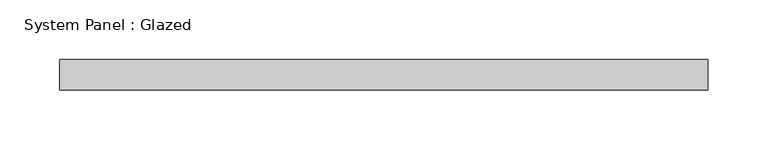
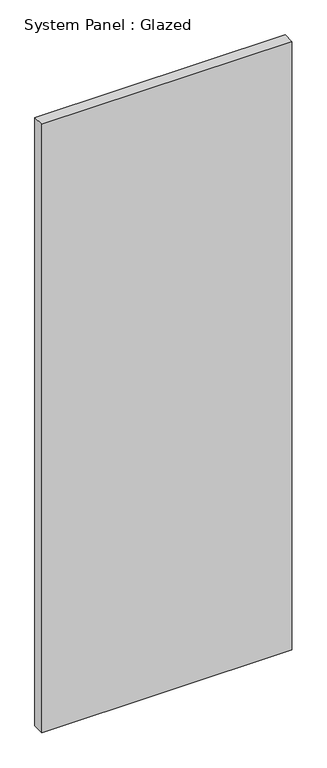
"""IFC4 building model written with IfcOpenShell, lengths in millimetres: plate geometry, System Panel : Glazed."""

from ifc_helpers import new_model, si_unit, origin, origin_with_axes, place, context, project, spatial, polyline, outline, extrude, source, transform, mapped, element, save


def system_panel_glazed_c810d226(model_context):
    return source(origin(), model_context, "Body", "SweptSolid", [
        extrude(outline(polyline([(271.258278, 19.05), (-271.258278, 19.05), (-271.258278, 44.45), (271.258278, 44.45), (271.258278, 19.05)])), origin_with_axes(), (0.0, 0.0, 1.0), 1394.9137173),
    ])


if __name__ == "__main__":
    model = new_model("IFC4")
    model_context = context("Model", 3, world=origin())
    ifc_project = project(units=[si_unit("LENGTHUNIT", "METRE", prefix="MILLI")], contexts=[model_context])
    site = spatial("IfcSite", under=ifc_project)
    building = spatial("IfcBuilding", under=site)
    placement = place(None, origin())
    system_panel_glazed_shape = system_panel_glazed_c810d226(model_context)
    element("IfcPlate", 1, ObjectType="System Panel : Glazed", at=placement, inside=building, context=model_context, shape_type="MappedRepresentation", body=[
        mapped(system_panel_glazed_shape, transform((0.0, 0.0, 0.0), x_axis=(1.0, 0.0, 0.0), y_axis=(0.0, 1.0, 0.0), z_axis=(0.0, 0.0, 1.0))),
    ])
    save(model, "model.ifc")

# Revit data of these elements
# Type "System Panel : Glazed"
#   Construction Type Id = "GSP4R"
#   Analytic Construction = "1/8 in Pilkington single glazing"
#   Visual Light Transmittance = 0.9
#   Solar Heat Gain Coefficient = 0.86
#   Heat Transfer Coefficient (U) = 1.18115 BTU/(h·ft²·°F)
#   Define Thermal Properties by = 1
# Element 1 (IfcPlate, "System Panel : Glazed")
#   Materials on its faces: "Glass"
# Materials
#   "Glass": class "Glass", colour RGB 0 128 192, transparency 0.75, Description = "Soda Lime Glass", Cost = 0
